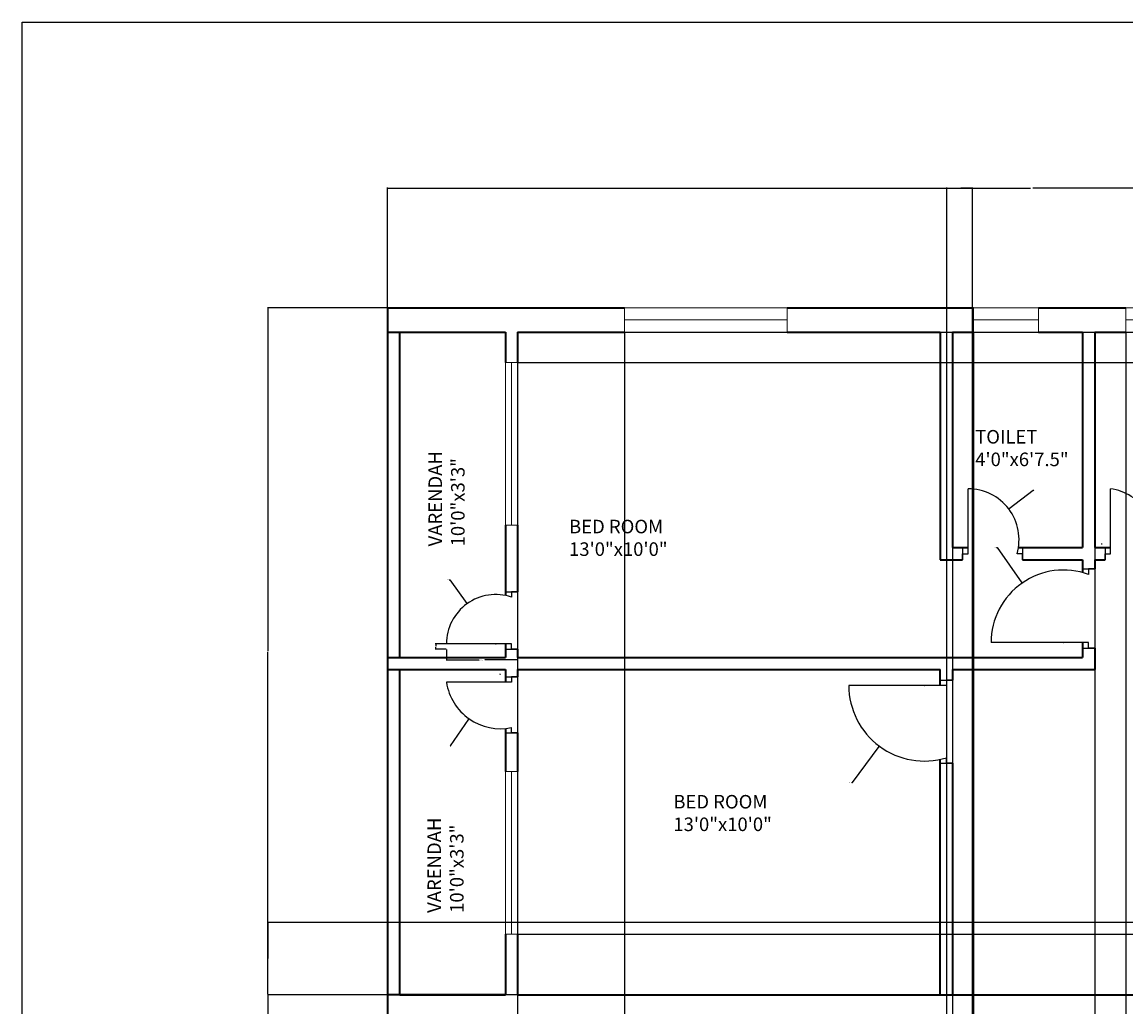
# Model space of a CAD drawing. Units: inches. Extents: x 1870 to 2611, y 1432 to 2511.
# Tile 4 of 5: x 1870 to 2277, y 2147 to 2511. Entities that reach past the tile are written whole.
import ezdxf

# ---------------------------------------------------------------- set-up
doc = ezdxf.new("R2010")
doc.units = ezdxf.units.IN
for name, color, linetype, lineweight in [('A-ANNO-DIMS', 2, 'Continuous', 18), ('A-ANNO-TTLB', 7, 'Continuous', 25), ('A-AREA-IDEN', 7, 'Continuous', 18), ('A-DOOR', 31, 'Continuous', 25), ('A-GLAZ', 201, 'Continuous', 18), ('A-WALL', 7, 'Continuous', 35)]:
    doc.layers.add(name, color=color, linetype=linetype, lineweight=lineweight)
doc.styles.get("Standard").update_dxf_attribs({"font": 'arial.ttf'})
doc.dimstyles.get("Standard").update_dxf_attribs({"dimtxt": 0.18, "dimasz": 0.18, "dimexe": 0.18, "dimexo": 0.0625, "dimgap": 0.09, "dimtad": 0, "dimtih": 1, "dimtoh": 1, "dimdec": 4, "dimzin": 0, "dimdsep": 46, "dimtxsty": 'Standard', "dimcen": 0.09, "dimadec": 0, "dimazin": 0, "dimtfac": 1, "dimtdec": 4, "dimtofl": 0, "dimtmove": 0, "dimatfit": 3, "dimfxl": 1, "dimtolj": 1, "dimtzin": 0, "dimarcsym": 0})

# ---------------------------------------------------------------- blocks, each defined once
blk = doc.blocks.new('DOOR-LEAF-36-JAMB-4P5')
for p, q in [((36, 2), (0, 2)), ((33.75, 0), (38.25, 0)), ((36, 0), (36, 2)), ((38.25, 0), (36, 0))]:
    blk.add_line(p, q)
blk = doc.blocks.new('DOOR-LEAF-24-JAMB-4P5')
for p, q in [((2, 2.25), (2, 26.25)), ((0, 4.5), (0, 0)), ((0, 0), (0, 2.25)), ((0, 2.25), (2, 2.25))]:
    blk.add_line(p, q)
blk = doc.blocks.new('WIN-60-FRAME-9')
for p, q in [((0, 9), (0, 0)), ((60, 9), (0, 9)), ((60, 4.5), (60, 9)), ((60, 9), (60, 0)), ((0, 0), (0, 4.5)), ((0, 4.5), (60, 4.5)), ((0, 0), (60, 0))]:
    blk.add_line(p, q)
blk = doc.blocks.new('WIN-24-FRAME-9')
for p, q in [((0, 9), (0, 0)), ((24, 9), (0, 9)), ((24, 4.5), (24, 9)), ((24, 9), (24, 0)), ((0, 0), (0, 4.5)), ((0, 4.5), (24, 4.5)), ((0, 0), (24, 0))]:
    blk.add_line(p, q)
blk = doc.blocks.new('WIN-60-FRAME-4P5')
for p, q in [((0, 60), (4.5, 60)), ((0, 60), (0, 0)), ((4.5, 60), (2.25, 60)), ((2.25, 60), (2.25, 0)), ((4.5, 60), (4.5, 0)), ((2.25, 0), (0, 0)), ((0, 0), (4.5, 0))]:
    blk.add_line(p, q)
blk = doc.blocks.new('*D9')
at = {"layer": 'A-ANNO-DIMS', "color": 0, "lineweight": -2, "transparency": 16777216}
for p, q in [((2026.39, 2279.28), (2026.39, 2275.22)), ((2052.64, 2279.28), (2052.64, 2275.22)), ((2026.57, 2275.4), (2038.46, 2275.4)), ((2052.46, 2275.4), (2040.57, 2275.4))]:
    blk.add_line(p, q, dxfattribs=at)
at = {"layer": 'A-ANNO-DIMS', "color": 0, "transparency": 16777216}
for points in [[(2026.57, 2275.43), (2026.57, 2275.37), (2026.39, 2275.4)], [(2052.46, 2275.43), (2052.46, 2275.37), (2052.64, 2275.4)]]:
    blk.add_solid(points, dxfattribs=at)
at = {"layer": 'Defpoints', "color": 0, "transparency": 16777216}
for p in [(2026.39, 2279.34), (2052.64, 2279.34), (2026.39, 2275.4)]:
    blk.add_point(p, dxfattribs=at)
at = {"layer": 'A-ANNO-DIMS', "color": 0, "transparency": 16777216, "insert": (2039.51, 2275.4), "char_height": 0.18, "attachment_point": 5}
blk.add_mtext('\\A1;DOOR A 26 TYP.', dxfattribs=at)
blk = doc.blocks.new('*D10')
at = {"layer": 'A-ANNO-DIMS', "color": 0, "lineweight": -2, "transparency": 16777216}
for p, q in [((2026.32, 2281.34), (2022.27, 2281.34)), ((2026.32, 2279.34), (2022.27, 2279.34)), ((2022.45, 2281.16), (2022.45, 2280.52)), ((2022.45, 2279.52), (2022.45, 2280.16))]:
    blk.add_line(p, q, dxfattribs=at)
at = {"layer": 'A-ANNO-DIMS', "color": 0, "transparency": 16777216}
for points in [[(2022.42, 2281.16), (2022.48, 2281.16), (2022.45, 2281.34)], [(2022.42, 2279.52), (2022.48, 2279.52), (2022.45, 2279.34)]]:
    blk.add_solid(points, dxfattribs=at)
at = {"layer": 'Defpoints', "color": 0, "transparency": 16777216}
for p in [(2022.45, 2281.34), (2026.39, 2281.34), (2026.39, 2279.34)]:
    blk.add_point(p, dxfattribs=at)
at = {"layer": 'A-ANNO-DIMS', "color": 0, "transparency": 16777216, "insert": (2022.45, 2280.34), "char_height": 0.18, "attachment_point": 5}
blk.add_mtext('\\A1;2 TYP.', dxfattribs=at)
blk = doc.blocks.new('*D25')
at = {"layer": 'A-ANNO-DIMS', "color": 0, "lineweight": -2, "transparency": 16777216}
for p, q in [((2004.64, 2405.43), (2004.64, 2449.7)), ((2004.82, 2449.52), (2241.99, 2449.52)), ((2479.96, 2449.52), (2242.78, 2449.52)), ((2480.14, 2405.43), (2480.14, 2449.7))]:
    blk.add_line(p, q, dxfattribs=at)
at = {"layer": 'A-ANNO-DIMS', "color": 0, "transparency": 16777216}
for points in [[(2004.82, 2449.55), (2004.82, 2449.49), (2004.64, 2449.52)], [(2479.96, 2449.55), (2479.96, 2449.49), (2480.14, 2449.52)]]:
    blk.add_solid(points, dxfattribs=at)
at = {"layer": 'Defpoints', "color": 0, "transparency": 16777216}
for p in [(2480.14, 2449.52), (2004.64, 2405.37), (2480.14, 2405.37)]:
    blk.add_point(p, dxfattribs=at)
at = {"layer": 'A-ANNO-DIMS', "color": 0, "transparency": 16777216, "insert": (2242.39, 2449.52), "char_height": 0.18, "attachment_point": 5}
blk.add_mtext('\\A1;475.5', dxfattribs=at)
blk = doc.blocks.new('*D27')
at = {"layer": 'A-ANNO-DIMS', "color": 0, "lineweight": -2, "transparency": 16777216}
for p, q in [((2004.57, 2405.37), (1960.31, 2405.37)), ((1960.49, 2405.19), (1960.49, 2278.8)), ((1960.49, 2152.05), (1960.49, 2278.43)), ((2004.57, 2151.87), (1960.31, 2151.87))]:
    blk.add_line(p, q, dxfattribs=at)
at = {"layer": 'A-ANNO-DIMS', "color": 0, "transparency": 16777216}
for points in [[(1960.46, 2405.19), (1960.52, 2405.19), (1960.49, 2405.37)], [(1960.46, 2152.05), (1960.52, 2152.05), (1960.49, 2151.87)]]:
    blk.add_solid(points, dxfattribs=at)
at = {"layer": 'Defpoints', "color": 0, "transparency": 16777216}
for p in [(2004.64, 2405.37), (1960.49, 2151.87), (2004.64, 2151.87)]:
    blk.add_point(p, dxfattribs=at)
at = {"layer": 'A-ANNO-DIMS', "color": 0, "transparency": 16777216, "insert": (1960.49, 2278.62), "char_height": 0.18, "attachment_point": 5}
blk.add_mtext('\\A1;253.5', dxfattribs=at)
blk = doc.blocks.new('*D28')
at = {"layer": 'A-ANNO-DIMS', "color": 0, "lineweight": -2, "transparency": 16777216}
for p, q in [((2004.57, 2151.87), (1960.31, 2151.87)), ((1960.49, 2151.69), (1960.49, 2029.8)), ((1960.49, 1907.55), (1960.49, 2029.44)), ((2026.46, 1907.37), (1960.31, 1907.37))]:
    blk.add_line(p, q, dxfattribs=at)
at = {"layer": 'A-ANNO-DIMS', "color": 0, "transparency": 16777216}
for points in [[(1960.46, 2151.69), (1960.52, 2151.69), (1960.49, 2151.87)], [(1960.46, 1907.55), (1960.52, 1907.55), (1960.49, 1907.37)]]:
    blk.add_solid(points, dxfattribs=at)
at = {"layer": 'Defpoints', "color": 0, "transparency": 16777216}
for p in [(2004.64, 2151.87), (1960.49, 1907.37), (2026.52, 1907.37)]:
    blk.add_point(p, dxfattribs=at)
at = {"layer": 'A-ANNO-DIMS', "color": 0, "transparency": 16777216, "insert": (1960.49, 2029.62), "char_height": 0.18, "attachment_point": 5}
blk.add_mtext('\\A1;244.5', dxfattribs=at)
blk = doc.blocks.new('*D39')
at = {"layer": 'A-ANNO-DIMS', "color": 0, "lineweight": -2, "transparency": 16777216}
for p, q in [((2052.64, 2396.3), (2052.64, 1485.35)), ((2092.09, 2396.3), (2092.09, 1485.35)), ((2052.82, 1485.53), (2071.97, 1485.53)), ((2091.91, 1485.53), (2072.76, 1485.53))]:
    blk.add_line(p, q, dxfattribs=at)
at = {"layer": 'A-ANNO-DIMS', "color": 0, "transparency": 16777216}
for points in [[(2052.82, 1485.56), (2052.82, 1485.5), (2052.64, 1485.53)], [(2091.91, 1485.56), (2091.91, 1485.5), (2092.09, 1485.53)]]:
    blk.add_solid(points, dxfattribs=at)
at = {"layer": 'Defpoints', "color": 0, "transparency": 16777216}
for p in [(2052.64, 2396.37), (2092.09, 2396.37), (2092.09, 1485.53)]:
    blk.add_point(p, dxfattribs=at)
at = {"layer": 'A-ANNO-DIMS', "color": 0, "transparency": 16777216, "insert": (2072.36, 1485.53), "char_height": 0.18, "attachment_point": 5}
blk.add_mtext('\\A1;39.45', dxfattribs=at)
blk = doc.blocks.new('*D40')
at = {"layer": 'A-ANNO-DIMS', "color": 0, "lineweight": -2, "transparency": 16777216}
for p, q in [((2213.14, 2396.3), (2213.14, 1485.35)), ((2220.9, 2396.3), (2220.9, 1485.35)), ((2213.32, 1485.53), (2216.63, 1485.53)), ((2220.72, 1485.53), (2217.41, 1485.53))]:
    blk.add_line(p, q, dxfattribs=at)
at = {"layer": 'A-ANNO-DIMS', "color": 0, "transparency": 16777216}
for points in [[(2213.32, 1485.56), (2213.32, 1485.5), (2213.14, 1485.53)], [(2220.72, 1485.56), (2220.72, 1485.5), (2220.9, 1485.53)]]:
    blk.add_solid(points, dxfattribs=at)
at = {"layer": 'Defpoints', "color": 0, "transparency": 16777216}
for p in [(2213.14, 2396.37), (2220.9, 2396.37), (2220.9, 1485.53)]:
    blk.add_point(p, dxfattribs=at)
at = {"layer": 'A-ANNO-DIMS', "color": 0, "transparency": 16777216, "insert": (2217.02, 1485.53), "char_height": 0.18, "attachment_point": 5}
blk.add_mtext('\\A1;7.766', dxfattribs=at)
blk = doc.blocks.new('*D41')
at = {"layer": 'A-ANNO-DIMS', "color": 0, "lineweight": -2, "transparency": 16777216}
for p, q in [((2265.64, 2396.3), (2265.64, 1485.35)), ((2277.17, 2396.3), (2277.17, 1485.35)), ((2265.82, 1485.53), (2270.95, 1485.53)), ((2276.99, 1485.53), (2271.86, 1485.53))]:
    blk.add_line(p, q, dxfattribs=at)
at = {"layer": 'A-ANNO-DIMS', "color": 0, "transparency": 16777216}
for points in [[(2265.82, 1485.56), (2265.82, 1485.5), (2265.64, 1485.53)], [(2276.99, 1485.56), (2276.99, 1485.5), (2277.17, 1485.53)]]:
    blk.add_solid(points, dxfattribs=at)
at = {"layer": 'Defpoints', "color": 0, "transparency": 16777216}
for p in [(2265.64, 2396.37), (2277.17, 2396.37), (2277.17, 1485.53)]:
    blk.add_point(p, dxfattribs=at)
at = {"layer": 'A-ANNO-DIMS', "color": 0, "transparency": 16777216, "insert": (2271.4, 1485.53), "char_height": 0.18, "attachment_point": 5}
blk.add_mtext('\\A1;11.535', dxfattribs=at)
blk = doc.blocks.new('*D45')
at = {"layer": 'A-ANNO-DIMS', "color": 0, "lineweight": -2, "transparency": 16777216}
for p, q in [((2211.02, 1649.43), (2211.02, 2449.7)), ((2211.2, 2449.52), (2215.39, 2449.52)), ((2220.38, 2449.52), (2216.18, 2449.52)), ((2220.56, 1649.43), (2220.56, 2449.7))]:
    blk.add_line(p, q, dxfattribs=at)
at = {"layer": 'A-ANNO-DIMS', "color": 0, "transparency": 16777216}
for points in [[(2211.2, 2449.55), (2211.2, 2449.49), (2211.02, 2449.52)], [(2220.38, 2449.55), (2220.38, 2449.49), (2220.56, 2449.52)]]:
    blk.add_solid(points, dxfattribs=at)
at = {"layer": 'Defpoints', "color": 0, "transparency": 16777216}
for p in [(2220.56, 2449.52), (2211.02, 1649.37), (2220.56, 1649.37)]:
    blk.add_point(p, dxfattribs=at)
at = {"layer": 'A-ANNO-DIMS', "color": 0, "transparency": 16777216, "insert": (2215.79, 2449.52), "char_height": 0.18, "attachment_point": 5}
blk.add_mtext('\\A1;9.537', dxfattribs=at)
blk = doc.blocks.new('*D48')
at = {"layer": 'A-ANNO-DIMS', "color": 0, "lineweight": -2, "transparency": 16777216}
for p, q in [((2471.07, 2178.54), (1960.31, 2178.54)), ((1960.49, 2178.36), (1960.49, 2165.39)), ((1960.49, 2152.05), (1960.49, 2165.02)), ((2471.07, 2151.87), (1960.31, 2151.87))]:
    blk.add_line(p, q, dxfattribs=at)
at = {"layer": 'A-ANNO-DIMS', "color": 0, "transparency": 16777216}
for points in [[(1960.46, 2178.36), (1960.52, 2178.36), (1960.49, 2178.54)], [(1960.46, 2152.05), (1960.52, 2152.05), (1960.49, 2151.87)]]:
    blk.add_solid(points, dxfattribs=at)
at = {"layer": 'Defpoints', "color": 0, "transparency": 16777216}
for p in [(1960.49, 2178.54), (2471.14, 2178.54), (2471.14, 2151.87)]:
    blk.add_point(p, dxfattribs=at)
at = {"layer": 'A-ANNO-DIMS', "color": 0, "transparency": 16777216, "insert": (1960.49, 2165.2), "char_height": 0.18, "attachment_point": 5}
blk.add_mtext('\\A1;26.673', dxfattribs=at)
blk = doc.blocks.new('*D52')
at = {"layer": 'A-ANNO-DIMS', "color": 0, "lineweight": -2, "transparency": 16777216}
for p, q in [((2052.7, 2396.37), (2524.47, 2396.37)), ((2524.29, 2396.19), (2524.29, 2390.94)), ((2524.29, 2385.32), (2524.29, 2390.57)), ((2052.7, 2385.14), (2524.47, 2385.14))]:
    blk.add_line(p, q, dxfattribs=at)
at = {"layer": 'A-ANNO-DIMS', "color": 0, "transparency": 16777216}
for points in [[(2524.26, 2396.19), (2524.32, 2396.19), (2524.29, 2396.37)], [(2524.26, 2385.32), (2524.32, 2385.32), (2524.29, 2385.14)]]:
    blk.add_solid(points, dxfattribs=at)
at = {"layer": 'Defpoints', "color": 0, "transparency": 16777216}
for p in [(2052.64, 2396.37), (2524.29, 2396.37), (2052.64, 2385.14)]:
    blk.add_point(p, dxfattribs=at)
at = {"layer": 'A-ANNO-DIMS', "color": 0, "transparency": 16777216, "insert": (2524.29, 2390.76), "char_height": 0.18, "attachment_point": 5}
blk.add_mtext('\\A1;11.223', dxfattribs=at)
blk = doc.blocks.new('*D53')
at = {"layer": 'A-ANNO-DIMS', "color": 0, "lineweight": -2, "transparency": 16777216}
for p, q in [((2052.7, 2174.24), (2524.47, 2174.24)), ((2524.29, 2174.06), (2524.29, 2163.24)), ((2524.29, 2152.05), (2524.29, 2162.87)), ((2052.7, 2151.87), (2524.47, 2151.87))]:
    blk.add_line(p, q, dxfattribs=at)
at = {"layer": 'A-ANNO-DIMS', "color": 0, "transparency": 16777216}
for points in [[(2524.26, 2174.06), (2524.32, 2174.06), (2524.29, 2174.24)], [(2524.26, 2152.05), (2524.32, 2152.05), (2524.29, 2151.87)]]:
    blk.add_solid(points, dxfattribs=at)
at = {"layer": 'Defpoints', "color": 0, "transparency": 16777216}
for p in [(2052.64, 2174.24), (2524.29, 2174.24), (2052.64, 2151.87)]:
    blk.add_point(p, dxfattribs=at)
at = {"layer": 'A-ANNO-DIMS', "color": 0, "transparency": 16777216, "insert": (2524.29, 2163.05), "char_height": 0.18, "attachment_point": 5}
blk.add_mtext('\\A1;22.376', dxfattribs=at)
blk = doc.blocks.new('*D62')
at = {"layer": 'A-ANNO-DIMS', "color": 0, "lineweight": -2, "transparency": 16777216}
for p, q in [((2202.69, 2265.98), (2202.87, 2265.98)), ((2202.78, 2265.89), (2202.78, 2266.07)), ((2176.2, 2230.13), (2186.06, 2243.43)), ((2176.02, 2230.13), (2176.2, 2230.13))]:
    blk.add_line(p, q, dxfattribs=at)
at = {"layer": 'A-ANNO-DIMS', "color": 0, "transparency": 16777216}
blk.add_solid([(2186.04, 2243.45), (2186.08, 2243.41), (2186.17, 2243.58)], dxfattribs=at)
at = {"layer": 'Defpoints', "color": 0, "transparency": 16777216}
for p in [(2202.78, 2265.98), (2186.17, 2243.58)]:
    blk.add_point(p, dxfattribs=at)
at = {"layer": 'A-ANNO-DIMS', "color": 0, "transparency": 16777216, "insert": (2175.47, 2230.13), "char_height": 0.18, "attachment_point": 5}
blk.add_mtext('\\A1;R27.894', dxfattribs=at)
blk = doc.blocks.new('*D65')
at = {"layer": 'A-ANNO-DIMS', "color": 0, "lineweight": -2, "transparency": 16777216}
for p, q in [((2229.43, 2316.94), (2229.61, 2316.94)), ((2229.61, 2316.94), (2238.73, 2303.91)), ((2254.1, 2281.8), (2254.28, 2281.8)), ((2254.19, 2281.71), (2254.19, 2281.89))]:
    blk.add_line(p, q, dxfattribs=at)
at = {"layer": 'A-ANNO-DIMS', "color": 0, "transparency": 16777216}
blk.add_solid([(2238.75, 2303.93), (2238.7, 2303.89), (2238.83, 2303.76)], dxfattribs=at)
at = {"layer": 'Defpoints', "color": 0, "transparency": 16777216}
for p in [(2238.83, 2303.76), (2254.19, 2281.8)]:
    blk.add_point(p, dxfattribs=at)
at = {"layer": 'A-ANNO-DIMS', "color": 0, "transparency": 16777216, "insert": (2229.02, 2316.94), "char_height": 0.18, "attachment_point": 5}
blk.add_mtext('\\A1;R26.8', dxfattribs=at)
blk = doc.blocks.new('*D68')
at = {"layer": 'A-ANNO-DIMS', "color": 0, "lineweight": -2, "transparency": 16777216}
for p, q in [((2295.13, 2337.35), (2285.2, 2330.3)), ((2295.31, 2337.35), (2295.13, 2337.35)), ((2268.18, 2318.28), (2268.36, 2318.28)), ((2268.27, 2318.19), (2268.27, 2318.37))]:
    blk.add_line(p, q, dxfattribs=at)
at = {"layer": 'A-ANNO-DIMS', "color": 0, "transparency": 16777216}
blk.add_solid([(2285.19, 2330.33), (2285.22, 2330.28), (2285.06, 2330.2)], dxfattribs=at)
at = {"layer": 'Defpoints', "color": 0, "transparency": 16777216}
for p in [(2285.06, 2330.2), (2268.27, 2318.28)]:
    blk.add_point(p, dxfattribs=at)
at = {"layer": 'A-ANNO-DIMS', "color": 0, "transparency": 16777216, "insert": (2295.86, 2337.35), "char_height": 0.18, "attachment_point": 5}
blk.add_mtext('\\A1;R20.593', dxfattribs=at)
blk = doc.blocks.new('*D70')
at = {"layer": 'A-ANNO-DIMS', "color": 0, "lineweight": -2, "transparency": 16777216}
for p, q in [((2046.17, 2270.14), (2046.35, 2270.14)), ((2046.26, 2270.05), (2046.26, 2270.23)), ((2027.89, 2243.75), (2034.68, 2253.5)), ((2027.71, 2243.75), (2027.89, 2243.75))]:
    blk.add_line(p, q, dxfattribs=at)
at = {"layer": 'A-ANNO-DIMS', "color": 0, "transparency": 16777216}
blk.add_solid([(2034.65, 2253.51), (2034.7, 2253.48), (2034.78, 2253.64)], dxfattribs=at)
at = {"layer": 'Defpoints', "color": 0, "transparency": 16777216}
for p in [(2046.26, 2270.14), (2034.78, 2253.64)]:
    blk.add_point(p, dxfattribs=at)
at = {"layer": 'A-ANNO-DIMS', "color": 0, "transparency": 16777216, "insert": (2027.32, 2243.75), "char_height": 0.18, "attachment_point": 5}
blk.add_mtext('\\A1;R20.1', dxfattribs=at)
blk = doc.blocks.new('*D72')
at = {"layer": 'A-ANNO-DIMS', "color": 0, "lineweight": -2, "transparency": 16777216}
for p, q in [((2242.94, 2337.92), (2234.06, 2331.23)), ((2243.12, 2337.92), (2242.94, 2337.92)), ((2218.8, 2319.8), (2218.98, 2319.8)), ((2218.89, 2319.71), (2218.89, 2319.89))]:
    blk.add_line(p, q, dxfattribs=at)
at = {"layer": 'A-ANNO-DIMS', "color": 0, "transparency": 16777216}
blk.add_solid([(2234.05, 2331.26), (2234.08, 2331.21), (2233.92, 2331.13)], dxfattribs=at)
at = {"layer": 'Defpoints', "color": 0, "transparency": 16777216}
for p in [(2233.92, 2331.13), (2218.89, 2319.8)]:
    blk.add_point(p, dxfattribs=at)
at = {"layer": 'A-ANNO-DIMS', "color": 0, "transparency": 16777216, "insert": (2243.6, 2337.92), "char_height": 0.18, "attachment_point": 5}
blk.add_mtext('\\A1;R18.82', dxfattribs=at)
blk = doc.blocks.new('*D75')
at = {"layer": 'A-ANNO-DIMS', "color": 0, "lineweight": -2, "transparency": 16777216}
for p, q in [((2027.4, 2304.99), (2027.58, 2304.99)), ((2027.58, 2304.99), (2033.86, 2296.27)), ((2044.5, 2281.34), (2044.68, 2281.34)), ((2044.59, 2281.25), (2044.59, 2281.43))]:
    blk.add_line(p, q, dxfattribs=at)
at = {"layer": 'A-ANNO-DIMS', "color": 0, "transparency": 16777216}
blk.add_solid([(2033.88, 2296.28), (2033.83, 2296.25), (2033.96, 2296.12)], dxfattribs=at)
at = {"layer": 'Defpoints', "color": 0, "transparency": 16777216}
for p in [(2033.96, 2296.12), (2044.59, 2281.34)]:
    blk.add_point(p, dxfattribs=at)
at = {"layer": 'A-ANNO-DIMS', "color": 0, "transparency": 16777216, "insert": (2026.94, 2304.99), "char_height": 0.18, "attachment_point": 5}
blk.add_mtext('\\A1;R18.21', dxfattribs=at)

msp = doc.modelspace()

# ---------------------------------------------------------------- linework, layer by layer
at = {"layer": 'A-ANNO-TTLB'}
msp.add_lwpolyline([(1869.7418, 2510.8018), (2611.0646, 2510.8018), (2611.0646, 1431.531), (1869.7418, 1431.531)], close=True, dxfattribs=at)
at = {"layer": 'A-DOOR'}
for p, q in [((2238.9845, 2314.6169), (2236.9845, 2314.6169)), ((2238.9845, 2316.8669), (2238.9845, 2312.3669)), ((2238.9845, 2312.3669), (2238.9845, 2314.6169)), ((2269.4903, 2312.3669), (2269.4903, 2312.3669)), ((2261.1359, 2308.9741), (2265.6359, 2308.9741)), ((2265.6359, 2308.9741), (2263.3859, 2308.9741)), ((2263.3859, 2308.9741), (2263.3859, 2306.9741)), ((2048.1359, 2300.6009), (2052.6359, 2300.6009)), ((2052.6359, 2300.6009), (2050.3859, 2300.6009)), ((2050.3859, 2300.6009), (2050.3859, 2298.6009)), ((2050.3859, 2269.1751), (2050.3859, 2269.1751)), ((2050.3859, 2248.4685), (2050.3859, 2250.4685)), ((2048.1359, 2248.4685), (2052.6359, 2248.4685)), ((2052.6359, 2248.4685), (2050.3859, 2248.4685)), ((2208.6359, 2237.2927), (2213.1359, 2237.2927)), ((2210.8859, 2237.2927), (2210.8859, 2239.2927)), ((2213.1359, 2237.2927), (2210.8859, 2237.2927))]:
    msp.add_line(p, q, dxfattribs=at)
for centre, radius, start, end in [((2218.8923, 2319.7976), 18.8194, 344.021115, 90), ((2268.2662, 2318.2782), 20.5927, 349.758741, 80.992528), ((2254.1877, 2281.8001), 26.8018, 69.928419, 180), ((2044.5946, 2281.3378), 18.2087, 71.454745, 180), ((2046.2642, 2270.1395), 20.0982, 188.482012, 281.834024), ((2202.7804, 2265.9836), 27.8945, 180, 286.892503)]:
    msp.add_arc(centre, radius, start, end, dxfattribs=at)
at = {"layer": 'A-GLAZ'}
for p, q in [((2069.3934, 2405.3669), (2069.3934, 2405.3669)), ((2152.0868, 2405.3669), (2152.0868, 2405.3669)), ((2220.9018, 2396.3669), (2220.9018, 2405.3669)), ((2220.9018, 2405.3669), (2220.9018, 2400.8669)), ((2220.9018, 2405.3669), (2244.9018, 2405.3669)), ((2244.9018, 2400.8669), (2244.9018, 2405.3669)), ((2244.9018, 2405.3669), (2244.9018, 2396.3669)), ((2220.9018, 2400.8669), (2244.9018, 2400.8669)), ((2092.0868, 2396.3669), (2092.0868, 2396.3669)), ((2244.9018, 2396.3669), (2220.9018, 2396.3669)), ((2277.1709, 2396.3669), (2277.1709, 2396.3669)), ((2050.3859, 2385.1438), (2050.3859, 2385.1438))]:
    msp.add_line(p, q, dxfattribs=at)
at = {"layer": 'A-WALL'}
for p, q in [((2004.6359, 2405.3669), (2092.0868, 2405.3669)), ((2004.6359, 2405.3669), (2004.6359, 2132.9155)), ((2043.6359, 2405.3669), (2092.0868, 2405.3669)), ((2152.0868, 2405.3669), (2220.9018, 2405.3669)), ((2152.0868, 2405.3669), (2220.9018, 2405.3669)), ((2244.9018, 2405.3669), (2277.1709, 2405.3669)), ((2244.9018, 2405.3669), (2277.1709, 2405.3669)), ((2004.6359, 2396.3669), (2048.1359, 2396.3669)), ((2009.1359, 2396.3669), (2009.1359, 2396.3669)), ((2009.1359, 2276.3669), (2009.1359, 2396.3669)), ((2048.1359, 2396.3669), (2048.1359, 2385.1438)), ((2052.6359, 2396.3669), (2052.6359, 2385.1438)), ((2052.6359, 2396.3669), (2092.0868, 2396.3669)), ((2152.0868, 2396.3669), (2208.6359, 2396.3669)), ((2208.6359, 2396.3669), (2208.6359, 2312.3669)), ((2213.1359, 2396.3669), (2213.1359, 2316.8669)), ((2213.1359, 2396.3669), (2220.9018, 2396.3669)), ((2244.9018, 2396.3669), (2261.1359, 2396.3669)), ((2261.1359, 2396.3669), (2261.1359, 2316.8669)), ((2265.6359, 2396.3669), (2265.6359, 2316.8669)), ((2265.6359, 2396.3669), (2277.1709, 2396.3669)), ((2048.1359, 2325.1438), (2048.1359, 2299.1987)), ((2052.6359, 2325.1438), (2052.6359, 2300.6009)), ((2213.1359, 2316.8669), (2218.8923, 2316.8669)), ((2237.4821, 2316.8669), (2261.1359, 2316.8669)), ((2265.6359, 2316.8669), (2271.4903, 2316.8669)), ((2208.6359, 2312.3669), (2216.8923, 2312.3669)), ((2238.9845, 2312.3669), (2261.1359, 2312.3669)), ((2261.1359, 2312.3669), (2261.1359, 2307.6856)), ((2265.6359, 2312.3669), (2269.4903, 2312.3669)), ((2265.6359, 2312.3669), (2265.6359, 2308.9741)), ((2261.1359, 2281.8001), (2261.1359, 2276.3669)), ((2048.1359, 2281.3378), (2048.1359, 2276.3669)), ((2052.6359, 2279.3378), (2052.6359, 2276.3669)), ((2265.6359, 2279.8001), (2265.6359, 2271.8669)), ((2004.6359, 2276.3669), (2048.1359, 2276.3669)), ((2052.6359, 2276.3669), (2261.1359, 2276.3669)), ((2004.6359, 2271.8669), (2048.1359, 2271.8669)), ((2009.1359, 2151.8669), (2009.1359, 2271.8669)), ((2048.1359, 2271.8669), (2048.1359, 2267.1751)), ((2052.6359, 2271.8669), (2052.6359, 2269.1751)), ((2052.6359, 2271.8669), (2208.6359, 2271.8669)), ((2208.6359, 2265.9836), (2208.6359, 2271.8669)), ((2213.1359, 2271.8669), (2213.1359, 2267.9836)), ((2213.1359, 2271.8669), (2265.6359, 2271.8669)), ((2048.1359, 2250.1287), (2048.1359, 2234.2429)), ((2052.6359, 2248.4685), (2052.6359, 2234.2429)), ((2208.6359, 2151.8669), (2208.6359, 2238.7106)), ((2213.1359, 2237.2927), (2213.1359, 2151.8669)), ((2048.1359, 2174.2429), (2048.1359, 2151.8669)), ((2052.6359, 2174.2429), (2052.6359, 2151.8669)), ((2048.1359, 2151.8669), (2004.6359, 2151.8669)), ((2009.1359, 2151.8669), (2048.1359, 2151.8669)), ((2052.6359, 2151.8669), (2322.6359, 2151.8669)), ((2052.6359, 2151.8669), (2208.6359, 2151.8669))]:
    msp.add_line(p, q, dxfattribs=at)

# ---------------------------------------------------------------- block references
at = {"layer": 'A-DOOR'}
for name, p in [('DOOR-LEAF-24-JAMB-4P5', (2216.892, 2312.367)), ('DOOR-LEAF-24-JAMB-4P5', (2269.49, 2312.367)), ('DOOR-LEAF-36-JAMB-4P5', (2227.386, 2279.8))]:
    msp.add_blockref(name, p, dxfattribs=at)
at = {"layer": 'A-DOOR', "rotation": 90.00000000000115}
msp.add_blockref('DOOR-LEAF-24-JAMB-4P5', (2052.6359, 2279.3375), dxfattribs=at)
at = {"layer": 'A-DOOR', "extrusion": (0, 0, -1), "zscale": -1}
for name, p, rotation in [('DOOR-LEAF-24-JAMB-4P5', (-2052.6359, 2269.1754), 269.9999999999999), ('DOOR-LEAF-36-JAMB-4P5', (-2174.886, 2267.9837), 180)]:
    msp.add_blockref(name, p, dxfattribs=dict(at, rotation=rotation))
at = {"layer": 'A-GLAZ'}
for name, p in [('WIN-60-FRAME-9', (2092.087, 2396.367)), ('WIN-24-FRAME-9', (2277.171, 2396.367)), ('WIN-60-FRAME-4P5', (2048.136, 2174.243))]:
    msp.add_blockref(name, p, dxfattribs=at)
at = {"layer": 'A-GLAZ', "rotation": 180}
msp.add_blockref('WIN-60-FRAME-4P5', (2052.6358, 2385.1437), dxfattribs=at)

# ---------------------------------------------------------------- texts
at = {"layer": 'A-AREA-IDEN', "char_height": 5, "attachment_point": 1}
for s, width, insert in [('TOILET\\P4\'0"x6\'7.5"', 44.100164, (2221.5358, 2360.2662)), ('BED ROOM\\P13\'0"x10\'0"', 95.681203, (2071.627, 2327.1419)), ('BED ROOM\\P13\'0"x10\'0"', 113.914202, (2110.1224, 2225.5908))]:
    msp.add_mtext_dynamic_manual_height_columns(s, width=width, gutter_width=12.5, heights=[0], dxfattribs=dict(at, insert=insert))
at = {"layer": 'A-AREA-IDEN', "char_height": 5, "attachment_point": 1, "rotation": 90}
for width, insert in [(45.405424, (2019.7425, 2317.3167)), (47.401549, (2019.3698, 2182.0745))]:
    msp.add_mtext_dynamic_manual_height_columns('VARENDAH\\P10\'0"x3\'3"', width=width, gutter_width=12.5, heights=[0], dxfattribs=dict(at, insert=insert))

# ---------------------------------------------------------------- dimensions: what is measured, and where the dimension line sits
at = {"layer": 'A-ANNO-DIMS'}
for base, p1, p2, override, picture, middle in [((2480.1359, 2449.5169), (2004.6359, 2405.3669), (2480.1359, 2405.3669), {"dimdec": 1, "dimlfac": 1, "dimrnd": 0, "dimzin": 0, "dimdsep": 46, "dimlunit": 2}, '*D25', (2242.3859, 2449.5169)), ((2220.55567, 2449.51694), (2211.01824, 1649.36694), (2220.55567, 1649.36694), {"dimdec": 3, "dimlfac": 1, "dimrnd": 0, "dimzin": 0, "dimdsep": 46, "dimlunit": 2}, '*D45', (2215.78695, 2449.51694)), ((2092.0868, 1485.5313), (2052.6359, 2396.3669), (2092.0868, 2396.3669), {"dimdec": 2, "dimlfac": 1, "dimrnd": 0, "dimzin": 0, "dimdsep": 46, "dimlunit": 2}, '*D39', (2072.3614, 1485.5313)), ((2220.9018, 1485.5313), (2213.1359, 2396.3669), (2220.9018, 2396.3669), {"dimdec": 3, "dimlfac": 1, "dimrnd": 0, "dimzin": 0, "dimdsep": 46, "dimlunit": 2}, '*D40', (2217.0189, 1485.5313)), ((2277.1709, 1485.5313), (2265.6359, 2396.3669), (2277.1709, 2396.3669), {"dimdec": 3, "dimlfac": 1, "dimrnd": 0, "dimzin": 0, "dimdsep": 46, "dimlunit": 2}, '*D41', (2271.4034, 1485.5313))]:
    dim = msp.add_linear_dim(base=base, p1=p1, p2=p2, dimstyle='Standard', override=override, dxfattribs=at)
    dim.commit()
    dim.dimension.update_dxf_attribs({"geometry": picture, "text_midpoint": middle})
for base, p1, p2, override, picture, middle in [((1960.4859, 2151.8669), (2004.6359, 2405.3669), (2004.6359, 2151.8669), {"dimdec": 1, "dimlfac": 1, "dimrnd": 0, "dimzin": 0, "dimdsep": 46, "dimlunit": 2}, '*D27', (1960.4859, 2278.6169)), ((2524.2859, 2396.3669), (2052.6359, 2385.1438), (2052.6359, 2396.3669), {"dimdec": 3, "dimlfac": 1, "dimrnd": 0, "dimzin": 0, "dimdsep": 46, "dimlunit": 2}, '*D52', (2524.2859, 2390.7554)), ((1960.4859, 2178.5402), (2471.1359, 2151.8669), (2471.1359, 2178.5402), {"dimdec": 3, "dimlfac": 1, "dimrnd": 0, "dimzin": 0, "dimdsep": 46, "dimlunit": 2}, '*D48', (1960.4859, 2165.2036)), ((2524.2859, 2174.2429), (2052.6359, 2151.8669), (2052.6359, 2174.2429), {"dimdec": 3, "dimlfac": 1, "dimrnd": 0, "dimzin": 0, "dimdsep": 46, "dimlunit": 2}, '*D53', (2524.2859, 2163.0549)), ((1960.4859, 1907.3669), (2004.6359, 2151.8669), (2026.5182, 1907.3669), {"dimdec": 1, "dimlfac": 1, "dimrnd": 0, "dimzin": 0, "dimdsep": 46, "dimlunit": 2}, '*D28', (1960.4859, 2029.6169))]:
    dim = msp.add_linear_dim(base=base, p1=p1, p2=p2, angle=90, dimstyle='Standard', override=override, dxfattribs=at)
    dim.commit()
    dim.dimension.update_dxf_attribs({"geometry": picture, "text_midpoint": middle})
for center, mpoint, override, picture, middle in [((2218.8923, 2319.7976), (2233.9201, 2331.126), {"dimdec": 2, "dimlfac": 1, "dimrnd": 0, "dimzin": 0, "dimdsep": 46, "dimlunit": 2}, '*D72', (2243.5956, 2337.9231)), ((2268.2662, 2318.2782), (2285.057, 2330.2), {"dimdec": 3, "dimlfac": 1, "dimrnd": 0, "dimzin": 0, "dimdsep": 46, "dimlunit": 2}, '*D68', (2295.8612, 2337.3531)), ((2254.1877, 2281.8001), (2238.8286, 2303.7645), {"dimdec": 1, "dimlfac": 1, "dimrnd": 0, "dimzin": 0, "dimdsep": 46, "dimlunit": 2}, '*D65', (2229.0231, 2316.9431)), ((2044.5946, 2281.3378), (2033.9622, 2296.1198), {"dimdec": 2, "dimlfac": 1, "dimrnd": 0, "dimzin": 0, "dimdsep": 46, "dimlunit": 2}, '*D75', (2026.9403, 2304.989)), ((2046.2642, 2270.1395), (2034.7821, 2253.6442), {"dimdec": 1, "dimlfac": 1, "dimrnd": 0, "dimzin": 0, "dimdsep": 46, "dimlunit": 2}, '*D70', (2027.3203, 2243.747)), ((2202.78042, 2265.983566), (2186.167018, 2243.576024), {"dimdec": 3, "dimlfac": 1, "dimrnd": 0, "dimzin": 0, "dimdsep": 46, "dimlunit": 2}, '*D62', (2175.469583, 2230.131498))]:
    dim = msp.add_radius_dim(center=center, mpoint=mpoint, dimstyle='Standard', override=override, dxfattribs=at)
    dim.commit()
    dim.dimension.update_dxf_attribs({"geometry": picture, "text_midpoint": middle, "dimtype": 164})
for base, p1, p2, angle, text, picture, middle in [((2022.4484, 2281.3378), (2026.3859, 2279.3378), (2026.3859, 2281.3378), 90, '<> TYP.', '*D10', (2022.4484, 2280.3378)), ((2026.3859, 2275.4003), (2052.6359, 2279.3378), (2026.3859, 2279.3378), 180, 'DOOR A <> TYP.', '*D9', (2039.5109, 2275.4003))]:
    dim = msp.add_linear_dim(base=base, p1=p1, p2=p2, angle=angle, text=text, dimstyle='Standard', override={"dimdec": 0, "dimlfac": 1, "dimrnd": 0, "dimzin": 0, "dimdsep": 46, "dimlunit": 2}, dxfattribs=at)
    dim.commit()
    dim.dimension.update_dxf_attribs({"geometry": picture, "text_midpoint": middle})

doc.saveas('drawing.dxf')
